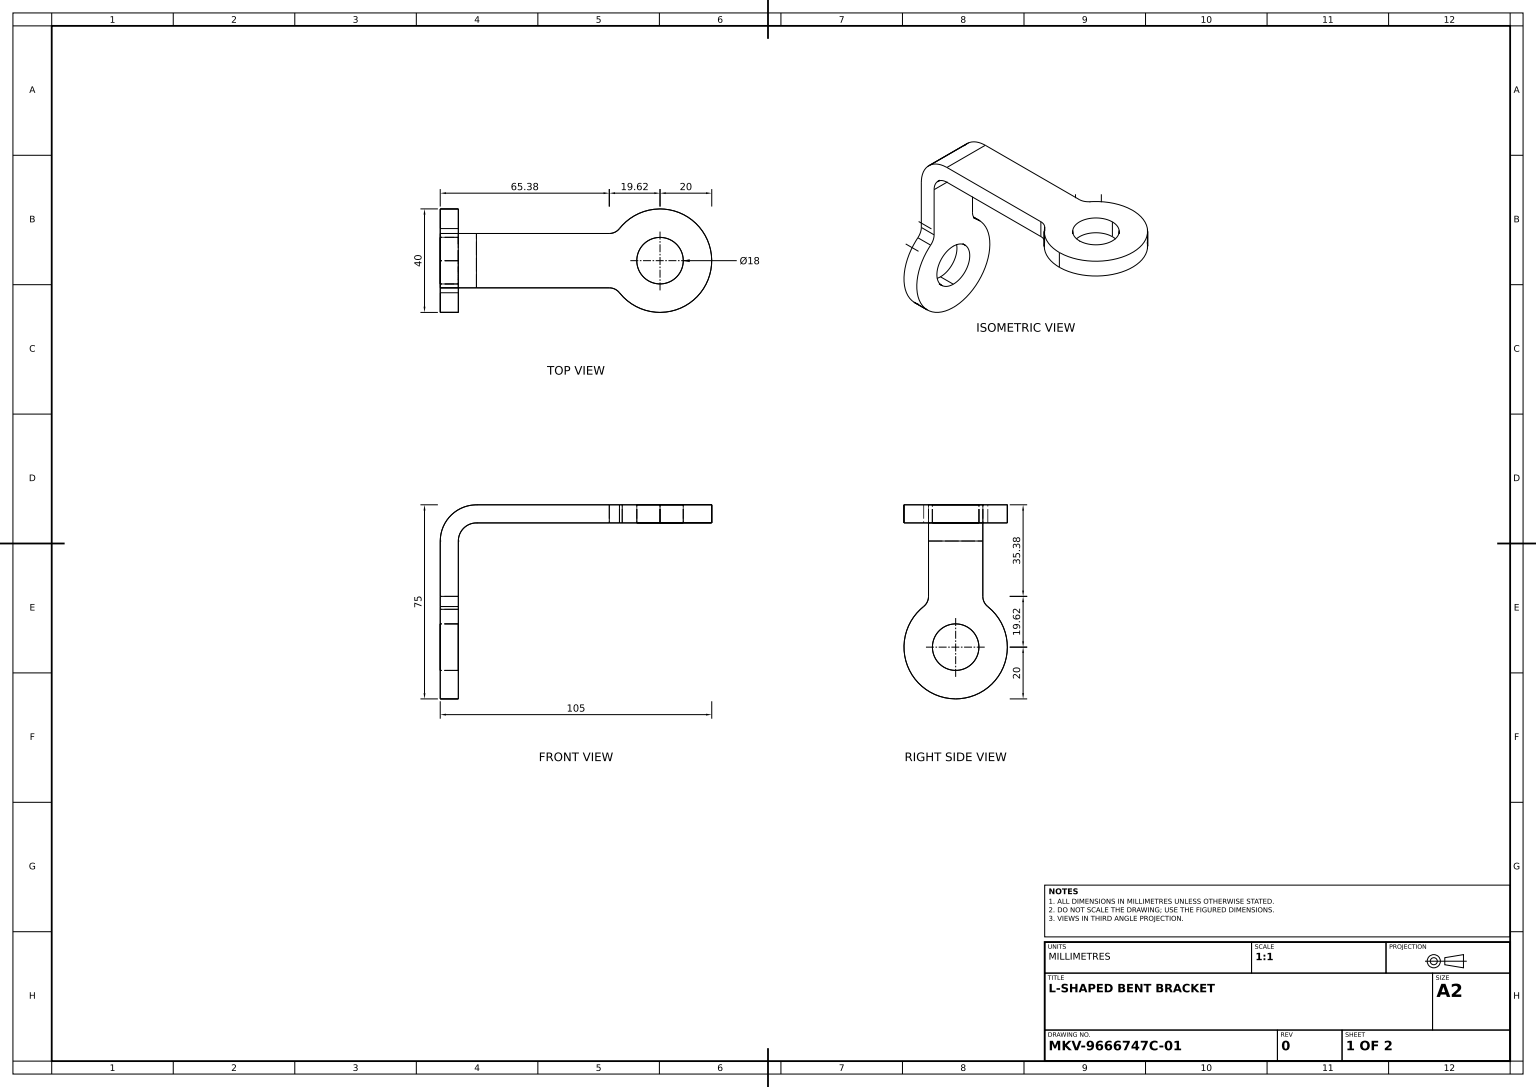
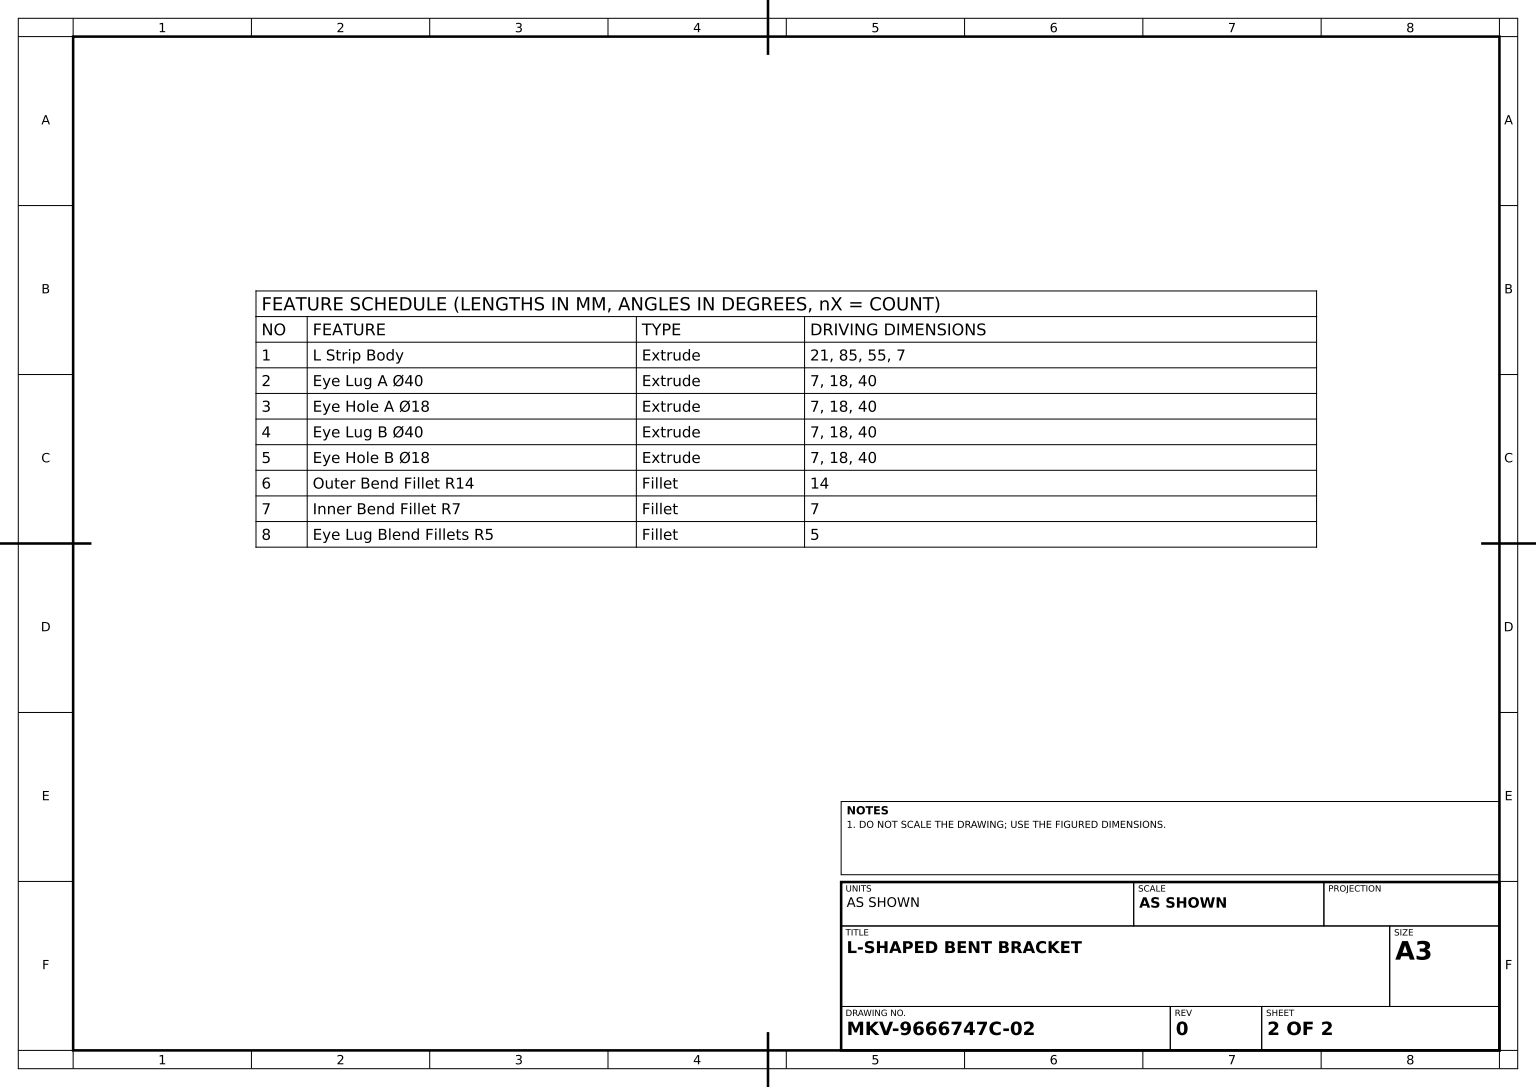
from build123d import *

# Parameters (mm, degrees)
L_STRIP_BODY_DEPTH         = 10.5
EYE_LUG_A_SKETCH_R         = 20
EYE_LUG_A_40_DEPTH         = 7
EYE_HOLE_A_18_DEPTH        = 7
EYE_LUG_B_SKETCH_R         = 20
EYE_LUG_B_SKETCH_R_2       = 9
EYE_LUG_B_40_DEPTH         = 7
EYE_HOLE_B_18_DEPTH        = 7
OUTER_BEND_FILLET_R14_R    = 14
INNER_BEND_FILLET_R7_R     = 7
EYE_LUG_BLEND_FILLETS_R5_R = 5


with BuildPart() as part:
    # L Strip Profile Sketch → L Strip Body (new, symmetric)
    with BuildSketch(Plane.XY):
        Polygon((85, 0), (0, 0), (0, -55), (7, -55), (7, -7), (85, -7), align=None)
    extrude(amount=L_STRIP_BODY_DEPTH, both=True)

    # Eye Lug A Sketch → Eye Lug A _40 (add)
    with BuildSketch(Plane(origin=(0, 0, 0), x_dir=(1, 0, 0), z_dir=(0, 1, 0))):
        with Locations((85, 0)):
            Circle(EYE_LUG_A_SKETCH_R)
    extrude(amount=-EYE_LUG_A_40_DEPTH)

    # Sketch2_3 → Eye Hole A _18 (cut)
    with BuildSketch(Plane(origin=(0, 0, 0), x_dir=(1, 0, 0), z_dir=(0, 1, 0))):
        with BuildLine():
            Line((85, 9), (85, -9))
            ThreePointArc((85, -9), (91.363961031, -6.363961031), (94, 0))
            ThreePointArc((94, 0), (91.363961031, 6.363961031), (85, 9))
        make_face()
        with BuildLine():
            ThreePointArc((85, 9), (76, 0), (85, -9))
            Line((85, -9), (85, 9))
        make_face()
        with BuildLine():
            Line((85, 9), (85, -9))
            ThreePointArc((85, -9), (91.363961031, -6.363961031), (94, 0))
            ThreePointArc((94, 0), (91.363961031, 6.363961031), (85, 9))
        make_face()
        with BuildLine():
            ThreePointArc((85, 9), (76, 0), (85, -9))
            Line((85, -9), (85, 9))
        make_face()
    extrude(amount=-EYE_HOLE_A_18_DEPTH, mode=Mode.SUBTRACT)

    # Eye Lug B Sketch → Eye Lug B _40 (add)
    with BuildSketch(Plane.ZY):
        with Locations((0, -55)):
            Circle(EYE_LUG_B_SKETCH_R)
        with Locations((0, -55)):
            Circle(EYE_LUG_B_SKETCH_R_2, mode=Mode.SUBTRACT)
    extrude(amount=-EYE_LUG_B_40_DEPTH)

    # Sketch4_2 → Eye Hole B _18 (cut)
    with BuildSketch(Plane.ZY):
        with BuildLine():
            Line((-9, -55), (9, -55))
            ThreePointArc((9, -55), (0, -46), (-9, -55))
        make_face()
        with BuildLine():
            ThreePointArc((-9, -55), (0, -64), (9, -55))
            Line((9, -55), (-9, -55))
        make_face()
    extrude(amount=-EYE_HOLE_B_18_DEPTH, mode=Mode.SUBTRACT)

    # Outer Bend Fillet R14
    outer_bend_fillet_r14_edges = [part.edges().sort_by_distance(p)[0] for p in [
        (0, 0, 0),
    ]]
    fillet(outer_bend_fillet_r14_edges, radius=OUTER_BEND_FILLET_R14_R)

    # Inner Bend Fillet R7
    inner_bend_fillet_r7_edges = [part.edges().sort_by_distance(p)[0] for p in [
        (7, -7, 0),
    ]]
    fillet(inner_bend_fillet_r7_edges, radius=INNER_BEND_FILLET_R7_R)

    # Eye Lug Blend Fillets R5
    eye_lug_blend_fillets_r5_edges = [part.edges().sort_by_distance(p)[0] for p in [
        (67.977955469, -3.5, 10.5),
        (67.977955469, -3.5, -10.5),
        (3.5, -37.977955469, -10.5),
        (3.5, -37.977955469, 10.5),
    ]]
    fillet(eye_lug_blend_fillets_r5_edges, radius=EYE_LUG_BLEND_FILLETS_R5_R)


solid = part.part
